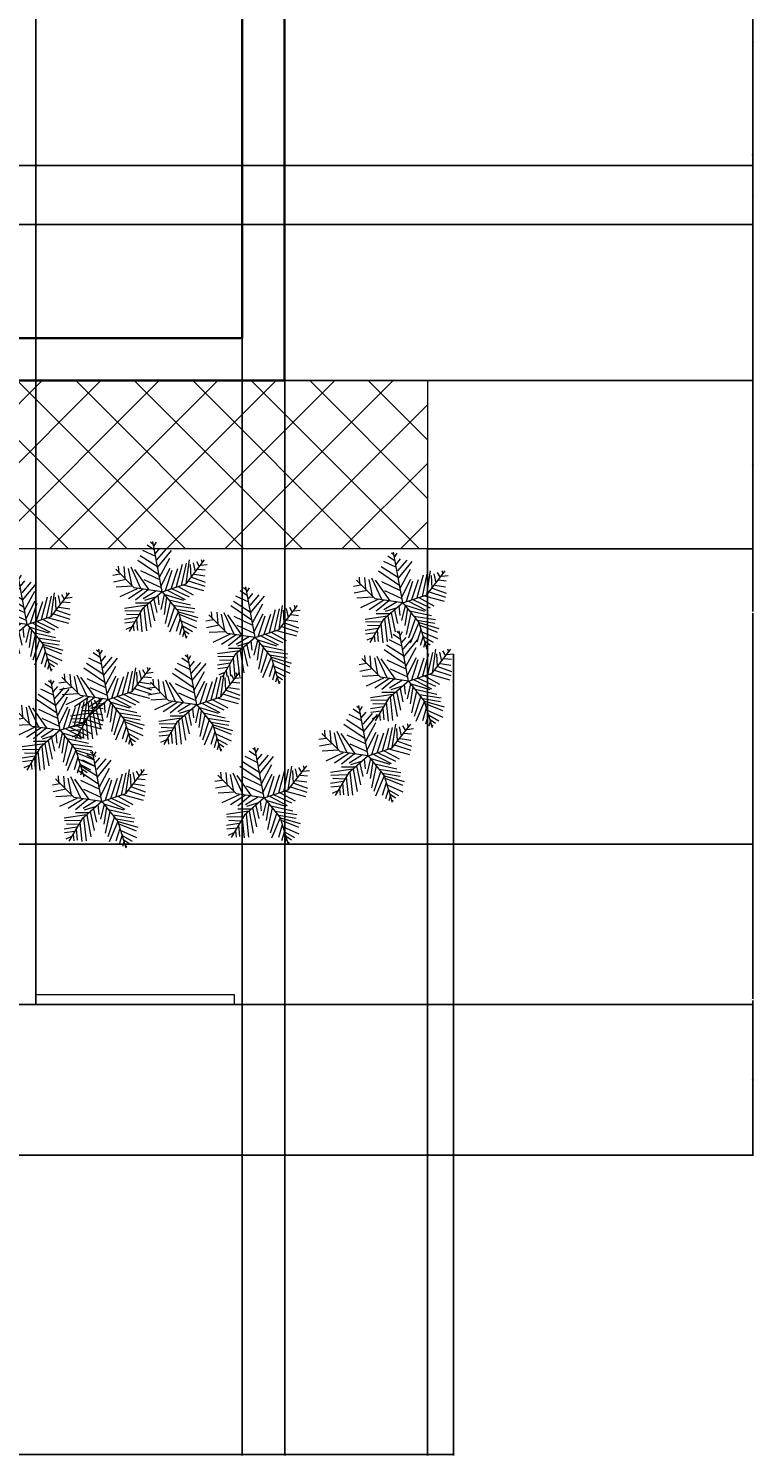
# Model space of a CAD drawing. Units: inches. Extents: x 818 to 1898, y 976 to 2364.
# Tile 18 of 96: x 1745 to 1898, y 976 to 1277. Entities that reach past the tile are written whole.
import ezdxf

# ---------------------------------------------------------------- set-up
doc = ezdxf.new("R2010")
doc.units = ezdxf.units.IN
doc.header["$LTSCALE"] = 5
doc.header["$MEASUREMENT"] = 0
for name, color, linetype, lineweight in [('A-ANNO-DIMS', 2, 'Continuous', 18), ('C-PAVE-PATT', 8, 'Continuous', 9), ('C-PROP', 7, 'Continuous', 35), ('C-ROAD', 8, 'Continuous', 25), ('C-ROAD-MRKG', 7, 'Continuous', 13), ('L-PAVE', 8, 'Continuous', 18)]:
    doc.layers.add(name, color=color, linetype=linetype, lineweight=lineweight)
doc.layers.add('L-PLNT', color=116, linetype='Continuous', lineweight=13, true_color=0x136734)
doc.styles.get("Standard").update_dxf_attribs({"font": 'arial.ttf'})
doc.dimstyles.get("Standard").update_dxf_attribs({"dimtxt": 0.18, "dimasz": 0.18, "dimexe": 0.18, "dimexo": 0.0625, "dimgap": 0.09, "dimtad": 0, "dimtih": 1, "dimtoh": 1, "dimdec": 4, "dimzin": 0, "dimdsep": 46, "dimtxsty": 'Standard', "dimcen": 0.09, "dimadec": 0, "dimazin": 0, "dimtfac": 1, "dimtdec": 4, "dimtofl": 0, "dimtmove": 0, "dimatfit": 3, "dimfxl": 1, "dimtolj": 1, "dimtzin": 0, "dimarcsym": 0})

# ---------------------------------------------------------------- blocks, each defined once
blk = doc.blocks.new('SHRUB-ACCENT')
for p, q in [((9.08, 17.24), (6.37, 18.54)), ((8.8, 18.63), (7.25, 19.67)), ((8.53, 19.84), (7.99, 20.28)), ((10.44, 9.82), (8.47, 20.47)), ((8.74, 19.5), (9.21, 20.28)), ((9.01, 17.93), (9.96, 19.06)), ((9.35, 16.54), (11.31, 18.8)), ((9.48, 14.98), (12.39, 18.54)), ((1.35, 13.77), (1.22, 15.24)), ((2.3, 15.16), (2.51, 12.72)), ((9.75, 13.42), (5.28, 16.46)), ((9.48, 15.07), (5.82, 17.41)), ((9.89, 12.9), (12.06, 16.89)), ((13.48, 10.9), (14.76, 15.68)), ((14.56, 11.16), (15.58, 15.85)), ((15.49, 11.5), (19.41, 16.55)), ((15.51, 11.51), (16.25, 16.54)), ((16.39, 15.59), (16.53, 12.9)), ((17, 15.94), (17.41, 14.03)), ((17.68, 16.2), (18.29, 15.16)), ((18.62, 15.42), (19.98, 15.59)), ((18.69, 16.63), (18.9, 15.94)), ((1.56, 13.51), (0, 13.25)), ((2.84, 12.38), (0.14, 11.86)), ((4.55, 10.66), (0.62, 14.58)), ((3.25, 14.72), (3.93, 11.25)), ((3.79, 15.07), (5.89, 10.55)), ((7.72, 10.21), (4.67, 14.55)), ((5.89, 14.29), (9.89, 12.38)), ((6.57, 12.38), (10.23, 10.73)), ((10.23, 11.07), (12.12, 14.81)), ((11.17, 10.12), (12.53, 14.37)), ((12.33, 10.47), (13.75, 14.72)), ((15.98, 12.12), (19.44, 10.99)), ((16.66, 12.9), (19.57, 11.86)), ((17.2, 13.51), (19.44, 13.16)), ((18.02, 14.63), (19.57, 14.46)), ((4.2, 10.99), (0.68, 10.81)), ((5.15, 10.47), (1.49, 8.73)), ((6.43, 10.38), (3.32, 8.3)), ((10.44, 9.82), (4.55, 10.66)), ((7.45, 10.21), (4.81, 8.04)), ((10.44, 9.82), (6.23, 6.17)), ((9.21, 10.03), (6.43, 8.3)), ((9.55, 9.16), (9.75, 7.08)), ((10.9, 9.25), (10.16, 6.04)), ((10.44, 9.82), (15.49, 11.5)), ((10.44, 9.82), (13.8, 5.61)), ((10.77, 9.34), (14.97, 8.04)), ((11.65, 10.12), (15.31, 8.21)), ((12.53, 10.47), (16.19, 8.73)), ((13.82, 10.9), (17, 9.16)), ((14.97, 11.25), (19.17, 10.12)), ((7.18, 6.99), (2.44, 6.3)), ((6.23, 6.17), (3.43, 1.4)), ((7.59, 7.43), (4.81, 7.43)), ((6.57, 6.39), (7.11, 1.52)), ((9.21, 8.73), (6.7, 7.95)), ((7.25, 6.99), (8.06, 2.31)), ((7.92, 7.69), (8.8, 3.69)), ((8.67, 8.21), (9.28, 5.43)), ((11.38, 8.64), (10.84, 5)), ((12.12, 7.69), (11.11, 3.09)), ((13.07, 6.65), (11.65, 2.31)), ((11.85, 8.12), (16.46, 7.08)), ((12.73, 6.99), (17.34, 6.3)), ((13.48, 6.13), (17.2, 5.52)), ((5.15, 4.39), (2.44, 3.95)), ((5.89, 5.78), (2.51, 5.69)), ((4.67, 3.43), (2.51, 3.17)), ((5.42, 4.91), (2.91, 5)), ((5.01, 4.04), (5.21, 1.61)), ((5.76, 5.34), (6.16, 1.35)), ((13.82, 5.6), (11.99, 1.26)), ((14.22, 4.13), (13.41, 1.44)), ((13.8, 5.61), (15.49, 0)), ((13.88, 5.6), (18.02, 4.39)), ((14.02, 5.08), (17.68, 3.61)), ((14.43, 3.69), (17.74, 2.22)), ((4, 2.39), (2.78, 1.87)), ((4.33, 2.91), (4.47, 1.52)), ((14.7, 2.74), (14.09, 0.74)), ((14.7, 2.65), (16.86, 1.44)), ((15.04, 1.26), (14.76, 0.31)), ((15.04, 1.7), (16.19, 0.92)), ((15.44, 0.48), (15.71, 0.31))]:
    blk.add_line(p, q)
blk = doc.blocks.new('LANE-STRIPE')
at = {"ltscale": 5}
for p, q in [((0, 2), (42, 2)), ((0, 2), (0, 0)), ((0, 0), (42, 0)), ((42, 2), (42, 0))]:
    blk.add_line(p, q, dxfattribs=at)
blk = doc.blocks.new('*D56')
at = {"layer": 'A-ANNO-DIMS', "color": 0, "lineweight": -2, "ltscale": 5, "transparency": 16777216}
for p, q in [((885.95, 1167.31), (885.95, 975.66)), ((1828.91, 1167.31), (1828.91, 975.66)), ((886.13, 975.84), (1357.14, 975.84)), ((1828.73, 975.84), (1357.72, 975.84))]:
    blk.add_line(p, q, dxfattribs=at)
at = {"layer": 'A-ANNO-DIMS', "color": 0, "ltscale": 5, "transparency": 16777216}
for points in [[(886.13, 975.87), (886.13, 975.81), (885.95, 975.84)], [(1828.73, 975.87), (1828.73, 975.81), (1828.91, 975.84)]]:
    blk.add_solid(points, dxfattribs=at)
at = {"layer": 'Defpoints', "color": 0, "ltscale": 5, "transparency": 16777216}
for p in [(885.95, 1167.37), (1828.91, 1167.37), (1828.91, 975.84)]:
    blk.add_point(p, dxfattribs=at)
at = {"layer": 'A-ANNO-DIMS', "color": 0, "ltscale": 5, "transparency": 16777216, "insert": (1357.43, 975.84), "char_height": 0.18, "attachment_point": 5}
blk.add_mtext('\\A1;943', dxfattribs=at)
blk = doc.blocks.new('*D58')
at = {"layer": 'A-ANNO-DIMS', "color": 0, "lineweight": -2, "ltscale": 5, "transparency": 16777216}
for p, q in [((881.51, 1159.31), (881.51, 975.66)), ((1834.44, 1145.13), (1834.44, 975.66)), ((881.69, 975.84), (1357.68, 975.84)), ((1834.26, 975.84), (1358.26, 975.84))]:
    blk.add_line(p, q, dxfattribs=at)
at = {"layer": 'A-ANNO-DIMS', "color": 0, "ltscale": 5, "transparency": 16777216}
for points in [[(881.69, 975.87), (881.69, 975.81), (881.51, 975.84)], [(1834.26, 975.87), (1834.26, 975.81), (1834.44, 975.84)]]:
    blk.add_solid(points, dxfattribs=at)
at = {"layer": 'Defpoints', "color": 0, "ltscale": 5, "transparency": 16777216}
for p in [(881.51, 1159.38), (1834.44, 1145.19), (1834.44, 975.84)]:
    blk.add_point(p, dxfattribs=at)
at = {"layer": 'A-ANNO-DIMS', "color": 0, "ltscale": 5, "transparency": 16777216, "insert": (1357.97, 975.84), "char_height": 0.18, "attachment_point": 5}
blk.add_mtext('\\A1;953', dxfattribs=at)
blk = doc.blocks.new('*D66')
at = {"layer": 'A-ANNO-DIMS', "color": 0, "lineweight": -2, "ltscale": 5, "transparency": 16777216}
for p, q in [((1714.73, 1346.02), (1714.73, 975.66)), ((1789.72, 1298.44), (1789.72, 975.66)), ((1714.91, 975.84), (1751.83, 975.84)), ((1789.54, 975.84), (1752.61, 975.84))]:
    blk.add_line(p, q, dxfattribs=at)
at = {"layer": 'A-ANNO-DIMS', "color": 0, "ltscale": 5, "transparency": 16777216}
for points in [[(1714.91, 975.87), (1714.91, 975.81), (1714.73, 975.84)], [(1789.54, 975.87), (1789.54, 975.81), (1789.72, 975.84)]]:
    blk.add_solid(points, dxfattribs=at)
at = {"layer": 'Defpoints', "color": 0, "ltscale": 5, "transparency": 16777216}
for p in [(1714.73, 1346.08), (1789.72, 1298.5), (1789.72, 975.84)]:
    blk.add_point(p, dxfattribs=at)
at = {"layer": 'A-ANNO-DIMS', "color": 0, "ltscale": 5, "transparency": 16777216, "insert": (1752.22, 975.84), "char_height": 0.18, "attachment_point": 5}
blk.add_mtext('\\A1;74.99', dxfattribs=at)
blk = doc.blocks.new('*D68')
at = {"layer": 'A-ANNO-DIMS', "color": 0, "lineweight": -2, "ltscale": 5, "transparency": 16777216}
for p, q in [((1828.97, 1104.97), (1897.92, 1104.97)), ((1897.74, 1104.79), (1897.74, 1072.24)), ((1897.74, 1039.32), (1897.74, 1071.87)), ((1828.97, 1039.14), (1897.92, 1039.14))]:
    blk.add_line(p, q, dxfattribs=at)
at = {"layer": 'A-ANNO-DIMS', "color": 0, "ltscale": 5, "transparency": 16777216}
for points in [[(1897.71, 1104.79), (1897.77, 1104.79), (1897.74, 1104.97)], [(1897.71, 1039.32), (1897.77, 1039.32), (1897.74, 1039.14)]]:
    blk.add_solid(points, dxfattribs=at)
at = {"layer": 'Defpoints', "color": 0, "ltscale": 5, "transparency": 16777216}
for p in [(1828.91, 1104.97), (1897.74, 1104.97), (1828.91, 1039.14)]:
    blk.add_point(p, dxfattribs=at)
at = {"layer": 'A-ANNO-DIMS', "color": 0, "ltscale": 5, "transparency": 16777216, "insert": (1897.74, 1072.06), "char_height": 0.18, "attachment_point": 5}
blk.add_mtext('\\A1;65.82', dxfattribs=at)
blk = doc.blocks.new('*D69')
at = {"layer": 'A-ANNO-DIMS', "color": 0, "lineweight": -2, "ltscale": 5, "transparency": 16777216}
for p, q in [((1798.78, 1202.96), (1897.92, 1202.96)), ((1897.74, 1202.78), (1897.74, 1154.15)), ((1897.74, 1105.15), (1897.74, 1153.78)), ((1828.97, 1104.97), (1897.92, 1104.97))]:
    blk.add_line(p, q, dxfattribs=at)
at = {"layer": 'A-ANNO-DIMS', "color": 0, "ltscale": 5, "transparency": 16777216}
for points in [[(1897.71, 1202.78), (1897.77, 1202.78), (1897.74, 1202.96)], [(1897.71, 1105.15), (1897.77, 1105.15), (1897.74, 1104.97)]]:
    blk.add_solid(points, dxfattribs=at)
at = {"layer": 'Defpoints', "color": 0, "ltscale": 5, "transparency": 16777216}
for p in [(1798.72, 1202.96), (1897.74, 1202.96), (1828.91, 1104.97)]:
    blk.add_point(p, dxfattribs=at)
at = {"layer": 'A-ANNO-DIMS', "color": 0, "ltscale": 5, "transparency": 16777216, "insert": (1897.74, 1153.97), "char_height": 0.18, "attachment_point": 5}
blk.add_mtext('\\A1;98', dxfattribs=at)
blk = doc.blocks.new('*D70')
at = {"layer": 'A-ANNO-DIMS', "color": 0, "lineweight": -2, "ltscale": 5, "transparency": 16777216}
for p, q in [((1714.79, 1346.08), (1897.92, 1346.08)), ((1897.74, 1345.9), (1897.74, 1274.7)), ((1897.74, 1203.14), (1897.74, 1274.34)), ((1798.78, 1202.96), (1897.92, 1202.96))]:
    blk.add_line(p, q, dxfattribs=at)
at = {"layer": 'A-ANNO-DIMS', "color": 0, "ltscale": 5, "transparency": 16777216}
for points in [[(1897.71, 1345.9), (1897.77, 1345.9), (1897.74, 1346.08)], [(1897.71, 1203.14), (1897.77, 1203.14), (1897.74, 1202.96)]]:
    blk.add_solid(points, dxfattribs=at)
at = {"layer": 'Defpoints', "color": 0, "ltscale": 5, "transparency": 16777216}
for p in [(1714.73, 1346.08), (1897.74, 1346.08), (1798.72, 1202.96)]:
    blk.add_point(p, dxfattribs=at)
at = {"layer": 'A-ANNO-DIMS', "color": 0, "ltscale": 5, "transparency": 16777216, "insert": (1897.74, 1274.52), "char_height": 0.18, "attachment_point": 5}
blk.add_mtext('\\A1;143.1', dxfattribs=at)
blk = doc.blocks.new('*D78')
at = {"layer": 'A-ANNO-DIMS', "color": 0, "lineweight": -2, "ltscale": 5, "transparency": 16777216}
for p, q in [((1798.72, 1202.9), (1798.72, 975.66)), ((1828.91, 1104.9), (1828.91, 975.66)), ((1798.9, 975.84), (1813.35, 975.84)), ((1828.73, 975.84), (1814.28, 975.84))]:
    blk.add_line(p, q, dxfattribs=at)
at = {"layer": 'A-ANNO-DIMS', "color": 0, "ltscale": 5, "transparency": 16777216}
for points in [[(1798.9, 975.87), (1798.9, 975.81), (1798.72, 975.84)], [(1828.73, 975.87), (1828.73, 975.81), (1828.91, 975.84)]]:
    blk.add_solid(points, dxfattribs=at)
at = {"layer": 'Defpoints', "color": 0, "ltscale": 5, "transparency": 16777216}
for p in [(1798.72, 1202.96), (1828.91, 1104.97), (1828.91, 975.84)]:
    blk.add_point(p, dxfattribs=at)
at = {"layer": 'A-ANNO-DIMS', "color": 0, "ltscale": 5, "transparency": 16777216, "insert": (1813.81, 975.84), "char_height": 0.18, "attachment_point": 5}
blk.add_mtext('\\A1;30.195', dxfattribs=at)
blk = doc.blocks.new('*D89')
at = {"layer": 'A-ANNO-DIMS', "color": 0, "lineweight": -2, "ltscale": 5, "transparency": 16777216}
for p, q in [((905.01, 1071.06), (1897.92, 1071.06)), ((1897.74, 1070.88), (1897.74, 1055.28)), ((1897.74, 1039.32), (1897.74, 1054.92)), ((896.18, 1039.14), (1897.92, 1039.14))]:
    blk.add_line(p, q, dxfattribs=at)
at = {"layer": 'A-ANNO-DIMS', "color": 0, "ltscale": 5, "transparency": 16777216}
for points in [[(1897.71, 1070.88), (1897.77, 1070.88), (1897.74, 1071.06)], [(1897.71, 1039.32), (1897.77, 1039.32), (1897.74, 1039.14)]]:
    blk.add_solid(points, dxfattribs=at)
at = {"layer": 'Defpoints', "color": 0, "ltscale": 5, "transparency": 16777216}
for p in [(904.95, 1071.06), (1897.74, 1071.06), (896.11, 1039.14)]:
    blk.add_point(p, dxfattribs=at)
at = {"layer": 'A-ANNO-DIMS', "color": 0, "ltscale": 5, "transparency": 16777216, "insert": (1897.74, 1055.1), "char_height": 0.18, "attachment_point": 5}
blk.add_mtext('\\A1;31.91', dxfattribs=at)
blk = doc.blocks.new('*D104')
at = {"layer": 'A-ANNO-DIMS', "color": 0, "lineweight": -2, "ltscale": 5, "transparency": 16777216}
for p, q in [((1689.47, 1071.12), (1689.47, 2363.87)), ((1689.65, 2363.69), (1717.4, 2363.69)), ((1745.9, 2363.69), (1718.15, 2363.69)), ((1746.08, 1071.12), (1746.08, 2363.87))]:
    blk.add_line(p, q, dxfattribs=at)
at = {"layer": 'A-ANNO-DIMS', "color": 0, "ltscale": 5, "transparency": 16777216}
for points in [[(1689.65, 2363.72), (1689.65, 2363.66), (1689.47, 2363.69)], [(1745.9, 2363.72), (1745.9, 2363.66), (1746.08, 2363.69)]]:
    blk.add_solid(points, dxfattribs=at)
at = {"layer": 'Defpoints', "color": 0, "ltscale": 5, "transparency": 16777216}
for p in [(1746.08, 2363.69), (1689.47, 1071.06), (1746.08, 1071.06)]:
    blk.add_point(p, dxfattribs=at)
at = {"layer": 'A-ANNO-DIMS', "color": 0, "ltscale": 5, "transparency": 16777216, "insert": (1717.78, 2363.69), "char_height": 0.18, "attachment_point": 5}
blk.add_mtext('\\A1;56.61', dxfattribs=at)
blk = doc.blocks.new('*D110')
at = {"layer": 'A-ANNO-DIMS', "color": 0, "lineweight": -2, "ltscale": 5, "transparency": 16777216}
for p, q in [((1164.62, 1248.46), (1897.92, 1248.46)), ((1897.74, 1248.28), (1897.74, 1242.4)), ((1897.74, 1236.14), (1897.74, 1242.03)), ((1116.25, 1235.96), (1897.92, 1235.96))]:
    blk.add_line(p, q, dxfattribs=at)
at = {"layer": 'A-ANNO-DIMS', "color": 0, "ltscale": 5, "transparency": 16777216}
for points in [[(1897.71, 1248.28), (1897.77, 1248.28), (1897.74, 1248.46)], [(1897.71, 1236.14), (1897.77, 1236.14), (1897.74, 1235.96)]]:
    blk.add_solid(points, dxfattribs=at)
at = {"layer": 'Defpoints', "color": 0, "ltscale": 5, "transparency": 16777216}
for p in [(1164.56, 1248.46), (1116.19, 1235.96), (1897.74, 1235.96)]:
    blk.add_point(p, dxfattribs=at)
at = {"layer": 'A-ANNO-DIMS', "color": 0, "ltscale": 5, "transparency": 16777216, "insert": (1897.74, 1242.21), "char_height": 0.18, "attachment_point": 5}
blk.add_mtext('\\A1;12.498', dxfattribs=at)
blk = doc.blocks.new('*D114')
at = {"layer": 'A-ANNO-DIMS', "color": 0, "lineweight": -2, "ltscale": 5, "transparency": 16777216}
for p, q in [((1766.41, 1298.5), (1897.92, 1298.5)), ((1897.74, 1298.32), (1897.74, 1250.92)), ((1897.74, 1203.14), (1897.74, 1250.55)), ((1798.78, 1202.96), (1897.92, 1202.96))]:
    blk.add_line(p, q, dxfattribs=at)
at = {"layer": 'A-ANNO-DIMS', "color": 0, "ltscale": 5, "transparency": 16777216}
for points in [[(1897.71, 1298.32), (1897.77, 1298.32), (1897.74, 1298.5)], [(1897.71, 1203.14), (1897.77, 1203.14), (1897.74, 1202.96)]]:
    blk.add_solid(points, dxfattribs=at)
at = {"layer": 'Defpoints', "color": 0, "ltscale": 5, "transparency": 16777216}
for p in [(1766.35, 1298.5), (1897.74, 1298.5), (1798.72, 1202.96)]:
    blk.add_point(p, dxfattribs=at)
at = {"layer": 'A-ANNO-DIMS', "color": 0, "ltscale": 5, "transparency": 16777216, "insert": (1897.74, 1250.73), "char_height": 0.18, "attachment_point": 5}
blk.add_mtext('\\A1;95.54', dxfattribs=at)
blk = doc.blocks.new('*D152')
at = {"layer": 'A-ANNO-DIMS', "color": 0, "lineweight": -2, "ltscale": 5, "transparency": 16777216}
for p, q in [((1828.97, 1202.96), (1897.92, 1202.96)), ((1897.74, 1202.78), (1897.74, 1185.35)), ((1897.74, 1167.55), (1897.74, 1184.99)), ((1828.97, 1167.37), (1897.92, 1167.37))]:
    blk.add_line(p, q, dxfattribs=at)
at = {"layer": 'A-ANNO-DIMS', "color": 0, "ltscale": 5, "transparency": 16777216}
for points in [[(1897.71, 1202.78), (1897.77, 1202.78), (1897.74, 1202.96)], [(1897.71, 1167.55), (1897.77, 1167.55), (1897.74, 1167.37)]]:
    blk.add_solid(points, dxfattribs=at)
at = {"layer": 'Defpoints', "color": 0, "ltscale": 5, "transparency": 16777216}
for p in [(1828.91, 1202.96), (1897.74, 1202.96), (1828.91, 1167.37)]:
    blk.add_point(p, dxfattribs=at)
at = {"layer": 'A-ANNO-DIMS', "color": 0, "ltscale": 5, "transparency": 16777216, "insert": (1897.74, 1185.17), "char_height": 0.18, "attachment_point": 5}
blk.add_mtext('\\A1;35.59', dxfattribs=at)

msp = doc.modelspace()

# ---------------------------------------------------------------- hatches: boundary and pattern name
at = {"layer": 'C-PAVE-PATT', "ltscale": 5}
h = msp.add_hatch(dxfattribs=at)
h.set_pattern_fill('ANSI37', color=256, scale=70)
h.paths.add_polyline_path([(1071.7252, 1202.9642), (885.9457, 1202.9642), (885.9457, 1167.3717), (1059.7252, 1167.3717, 0.41421356), (1071.7252, 1179.3717)])
h.paths.add_polyline_path([(1828.9123, 1202.9642), (1430.7252, 1202.9642), (1430.7252, 1179.3717, 0.41421356), (1442.7252, 1167.3717), (1828.9123, 1167.3717)])

# ---------------------------------------------------------------- linework, layer by layer
at = {"layer": 'C-PROP', "ltscale": 5}
for p, q in [((1798.7173, 1202.9642), (1798.7173, 2294.2171)), ((1789.7173, 1211.9642), (1789.7173, 2285.2171)), ((1789.7173, 1211.9642), (1430.7252, 1211.9642)), ((1798.7173, 1202.9642), (992.7252, 1202.9642))]:
    msp.add_line(p, q, dxfattribs=at)
at = {"layer": 'C-ROAD', "ltscale": 5}
msp.add_lwpolyline([(1828.9123, 1104.9672), (896.1138, 1104.9672), (896.1138, 1039.1433), (1828.9123, 1039.1433)], close=True, dxfattribs=at)
at = {"layer": 'L-PAVE', "ltscale": 5}
msp.add_lwpolyline([(1430.7252, 1202.9642), (1828.9123, 1202.9642), (1828.9123, 1167.3717), (1442.7252, 1167.3717, -0.41421356), (1430.7252, 1179.3717)], format="xyb", close=True, dxfattribs=at)

# ---------------------------------------------------------------- block references
at = {"layer": 'C-ROAD-MRKG', "rotation": 180}
msp.add_blockref('LANE-STRIPE', (1788.0843, 1073.0554), dxfattribs=at)
at = {"layer": 'L-PLNT'}
for p in [(1762.3591, 1148.499), (1813.2989, 1146.1854), (1733.8019, 1141.5583), (1782.0404, 1138.8592), (1814.4566, 1129.605), (1750.9492, 1125.7074), (1769.6913, 1124.5923), (1740.7483, 1119.194), (1805.9667, 1113.7957), (1749.6241, 1104.1559), (1783.9699, 1104.9271)]:
    msp.add_blockref('SHRUB-ACCENT', p, dxfattribs=at)

# ---------------------------------------------------------------- dimensions: what is measured, and where the dimension line sits
at = {"layer": 'A-ANNO-DIMS', "ltscale": 5}
for base, p1, p2, override, picture, middle in [((1746.0831, 2363.6929), (1689.4714, 1071.0552), (1746.0831, 1071.0552), {"dimdec": 2, "dimlfac": 1, "dimrnd": 0, "dimzin": 0, "dimdsep": 46, "dimlunit": 2}, '*D104', (1717.7772, 2363.6929)), ((1789.7173, 975.8433), (1714.7251, 1346.0782), (1789.7173, 1298.5041), {"dimdec": 2, "dimlfac": 1, "dimrnd": 0, "dimzin": 0, "dimdsep": 46, "dimlunit": 2}, '*D66', (1752.2212, 975.8433)), ((1828.9123, 975.8433), (1798.7173, 1202.9642), (1828.9123, 1104.9672), {"dimdec": 3, "dimlfac": 1, "dimrnd": 0, "dimzin": 0, "dimdsep": 46, "dimlunit": 2}, '*D78', (1813.8148, 975.8433)), ((1828.9123, 975.8433), (885.9457, 1167.3717), (1828.9123, 1167.3717), {"dimdec": 0, "dimlfac": 1, "dimrnd": 0, "dimzin": 0, "dimdsep": 46, "dimlunit": 2}, '*D56', (1357.429, 975.8433)), ((1834.436, 975.8433), (881.5059, 1159.375), (1834.436, 1145.1942), {"dimdec": 0, "dimlfac": 1, "dimrnd": 0, "dimzin": 0, "dimdsep": 46, "dimlunit": 2}, '*D58', (1357.971, 975.8433))]:
    dim = msp.add_linear_dim(base=base, p1=p1, p2=p2, dimstyle='Standard', override=override, dxfattribs=at)
    dim.commit()
    dim.dimension.update_dxf_attribs({"geometry": picture, "text_midpoint": middle})
for base, p1, p2, override, picture, middle in [((1897.736, 1346.0782), (1798.7173, 1202.9642), (1714.7251, 1346.0782), {"dimdec": 1, "dimlfac": 1, "dimrnd": 0, "dimzin": 0, "dimdsep": 46, "dimlunit": 2}, '*D70', (1897.736, 1274.5212)), ((1897.736, 1298.5041), (1798.7173, 1202.9642), (1766.3524, 1298.5041), {"dimdec": 2, "dimlfac": 1, "dimrnd": 0, "dimzin": 0, "dimdsep": 46, "dimlunit": 2}, '*D114', (1897.736, 1250.7342)), ((1897.736, 1235.9642), (1164.5571, 1248.4622), (1116.1882, 1235.9642), {"dimdec": 3, "dimlfac": 1, "dimrnd": 0, "dimzin": 0, "dimdsep": 46, "dimlunit": 2}, '*D110', (1897.736, 1242.2132)), ((1897.736, 1202.9642), (1828.9123, 1104.9672), (1798.7173, 1202.9642), {"dimdec": 0, "dimlfac": 1, "dimrnd": 0, "dimzin": 0, "dimdsep": 46, "dimlunit": 2}, '*D69', (1897.736, 1153.9657)), ((1897.736, 1202.9642), (1828.9123, 1167.3717), (1828.9123, 1202.9642), {"dimdec": 2, "dimlfac": 1, "dimrnd": 0, "dimzin": 0, "dimdsep": 46, "dimlunit": 2}, '*D152', (1897.736, 1185.1679)), ((1897.736, 1104.9672), (1828.9123, 1039.1433), (1828.9123, 1104.9672), {"dimdec": 2, "dimlfac": 1, "dimrnd": 0, "dimzin": 0, "dimdsep": 46, "dimlunit": 2}, '*D68', (1897.736, 1072.0552)), ((1897.736, 1071.0552), (896.1138, 1039.1433), (904.9504, 1071.0552), {"dimdec": 2, "dimlfac": 1, "dimrnd": 0, "dimzin": 0, "dimdsep": 46, "dimlunit": 2}, '*D89', (1897.736, 1055.0992))]:
    dim = msp.add_linear_dim(base=base, p1=p1, p2=p2, angle=90, dimstyle='Standard', override=override, dxfattribs=at)
    dim.commit()
    dim.dimension.update_dxf_attribs({"geometry": picture, "text_midpoint": middle})

doc.saveas('drawing.dxf')
